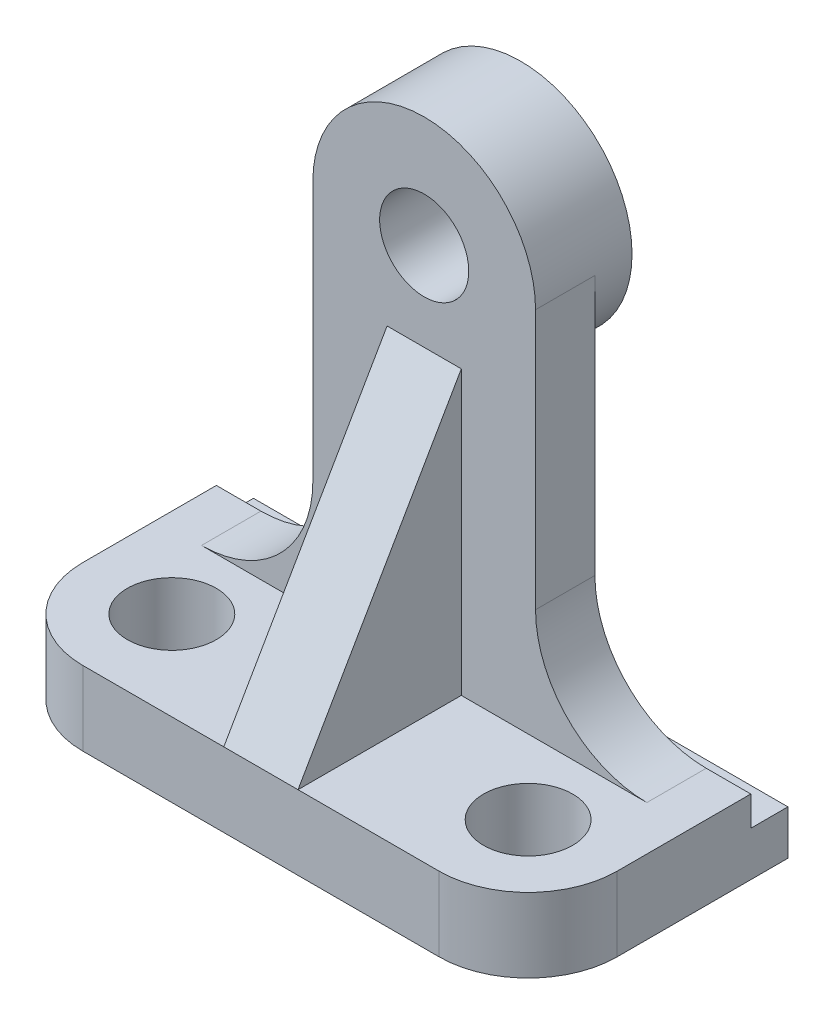
ISO-10303-21;
HEADER;
FILE_DESCRIPTION(('STEP AP214'),'2;1');
FILE_NAME('part.step','',(''),(''),'','','');
FILE_SCHEMA(('AUTOMOTIVE_DESIGN { 1 0 10303 214 1 1 1 1 }'));
ENDSEC;
DATA;
#1=APPLICATION_CONTEXT('core data for automotive mechanical design processes');
#2=APPLICATION_PROTOCOL_DEFINITION('international standard','automotive_design',2000,#1);
#3=PRODUCT_CONTEXT('',#1,'mechanical');
#4=PRODUCT('Part','Part','',(#3));
#5=PRODUCT_RELATED_PRODUCT_CATEGORY('part','',(#4));
#6=PRODUCT_DEFINITION_FORMATION('','',#4);
#7=PRODUCT_DEFINITION_CONTEXT('part definition',#1,'design');
#8=PRODUCT_DEFINITION('design','',#6,#7);
#9=PRODUCT_DEFINITION_SHAPE('','',#8);
#10=(LENGTH_UNIT() NAMED_UNIT(*) SI_UNIT(.MILLI.,.METRE.));
#11=(NAMED_UNIT(*) PLANE_ANGLE_UNIT() SI_UNIT($,.RADIAN.));
#12=(NAMED_UNIT(*) SI_UNIT($,.STERADIAN.) SOLID_ANGLE_UNIT());
#13=UNCERTAINTY_MEASURE_WITH_UNIT(LENGTH_MEASURE(1.E-05),#10,'distance_accuracy_value','');
#14=(GEOMETRIC_REPRESENTATION_CONTEXT(3) GLOBAL_UNCERTAINTY_ASSIGNED_CONTEXT((#13)) GLOBAL_UNIT_ASSIGNED_CONTEXT((#10,
#11,#12)) REPRESENTATION_CONTEXT('',''));
#15=CARTESIAN_POINT('',(0.,0.,0.));
#16=DIRECTION('',(0.,0.,1.));
#17=DIRECTION('',(1.,0.,0.));
#18=AXIS2_PLACEMENT_3D('',#15,#16,#17);
#19=CARTESIAN_POINT('',(23.9999999999999,10.,0.));
#20=DIRECTION('',(0.,-1.,0.));
#21=DIRECTION('',(0.,0.,-1.));
#22=AXIS2_PLACEMENT_3D('',#19,#20,#21);
#23=PLANE('',#22);
#24=CARTESIAN_POINT('',(-24.,10.,0.));
#25=DIRECTION('',(0.,1.,0.));
#26=DIRECTION('',(0.,0.,1.));
#27=AXIS2_PLACEMENT_3D('',#24,#25,#26);
#28=CIRCLE('',#27,6.);
#29=CARTESIAN_POINT('',(-24.,10.,6.));
#30=VERTEX_POINT('',#29);
#31=EDGE_CURVE('E250',#30,#30,#28,.T.);
#32=ORIENTED_EDGE('',*,*,#31,.F.);
#33=EDGE_LOOP('',(#32));
#34=FACE_BOUND('',#33,.T.);
#35=DIRECTION('',(0.,0.,1.));
#36=VECTOR('',#35,1.);
#37=CARTESIAN_POINT('',(-5.,10.,0.));
#38=LINE('',#37,#36);
#39=CARTESIAN_POINT('',(-5.,10.,-10.));
#40=VERTEX_POINT('',#39);
#41=CARTESIAN_POINT('',(-5.,10.,12.));
#42=VERTEX_POINT('',#41);
#43=EDGE_CURVE('E171',#40,#42,#38,.T.);
#44=ORIENTED_EDGE('',*,*,#43,.F.);
#45=DIRECTION('',(1.,0.,0.));
#46=VECTOR('',#45,1.);
#47=CARTESIAN_POINT('',(15.,10.,-10.));
#48=LINE('',#47,#46);
#49=CARTESIAN_POINT('',(-30.,10.,-10.));
#50=VERTEX_POINT('',#49);
#51=EDGE_CURVE('E158',#50,#40,#48,.T.);
#52=ORIENTED_EDGE('',*,*,#51,.F.);
#53=DIRECTION('',(0.,0.,-1.));
#54=VECTOR('',#53,1.);
#55=CARTESIAN_POINT('',(-30.,10.,-18.));
#56=LINE('',#55,#54);
#57=CARTESIAN_POINT('',(-30.,10.,-18.));
#58=VERTEX_POINT('',#57);
#59=EDGE_CURVE('E298',#50,#58,#56,.T.);
#60=ORIENTED_EDGE('',*,*,#59,.T.);
#61=DIRECTION('',(1.,0.,0.));
#62=VECTOR('',#61,1.);
#63=CARTESIAN_POINT('',(-36.,10.,-18.));
#64=LINE('',#63,#62);
#65=CARTESIAN_POINT('',(-36.,10.,-18.));
#66=VERTEX_POINT('',#65);
#67=EDGE_CURVE('E236',#66,#58,#64,.T.);
#68=ORIENTED_EDGE('',*,*,#67,.F.);
#69=DIRECTION('',(0.,0.,1.));
#70=VECTOR('',#69,1.);
#71=CARTESIAN_POINT('',(-36.,10.,-23.));
#72=LINE('',#71,#70);
#73=CARTESIAN_POINT('',(-36.,10.,0.));
#74=VERTEX_POINT('',#73);
#75=EDGE_CURVE('E258',#66,#74,#72,.T.);
#76=ORIENTED_EDGE('',*,*,#75,.T.);
#77=CARTESIAN_POINT('',(-24.,10.,0.));
#78=DIRECTION('',(0.,1.,0.));
#79=DIRECTION('',(0.,0.,-1.));
#80=AXIS2_PLACEMENT_3D('',#77,#78,#79);
#81=CIRCLE('',#80,12.);
#82=CARTESIAN_POINT('',(-24.,10.,12.));
#83=VERTEX_POINT('',#82);
#84=EDGE_CURVE('E259',#74,#83,#81,.T.);
#85=ORIENTED_EDGE('',*,*,#84,.T.);
#86=DIRECTION('',(1.,0.,0.));
#87=VECTOR('',#86,1.);
#88=CARTESIAN_POINT('',(-24.,10.,12.));
#89=LINE('',#88,#87);
#90=EDGE_CURVE('E174',#83,#42,#89,.T.);
#91=ORIENTED_EDGE('',*,*,#90,.T.);
#92=EDGE_LOOP('',(#44,#52,#60,#68,#76,#85,#91));
#93=FACE_BOUND('',#92,.T.);
#94=ADVANCED_FACE('F39',(#34,#93),#23,.F.);
#95=CARTESIAN_POINT('',(24.,10.,0.));
#96=DIRECTION('',(0.,1.,0.));
#97=DIRECTION('',(0.,0.,-1.));
#98=AXIS2_PLACEMENT_3D('',#95,#96,#97);
#99=CIRCLE('',#98,6.);
#100=CARTESIAN_POINT('',(24.,10.,-6.));
#101=VERTEX_POINT('',#100);
#102=EDGE_CURVE('E243',#101,#101,#99,.T.);
#103=ORIENTED_EDGE('',*,*,#102,.F.);
#104=EDGE_LOOP('',(#103));
#105=FACE_BOUND('',#104,.T.);
#106=CARTESIAN_POINT('',(5.,10.,-10.));
#107=VERTEX_POINT('',#106);
#108=CARTESIAN_POINT('',(30.,10.,-10.));
#109=VERTEX_POINT('',#108);
#110=EDGE_CURVE('E168',#107,#109,#48,.T.);
#111=ORIENTED_EDGE('',*,*,#110,.F.);
#112=DIRECTION('',(0.,0.,1.));
#113=VECTOR('',#112,1.);
#114=CARTESIAN_POINT('',(5.,10.,0.));
#115=LINE('',#114,#113);
#116=CARTESIAN_POINT('',(5.,10.,12.));
#117=VERTEX_POINT('',#116);
#118=EDGE_CURVE('E53',#107,#117,#115,.T.);
#119=ORIENTED_EDGE('',*,*,#118,.T.);
#120=CARTESIAN_POINT('',(24.,10.,12.));
#121=VERTEX_POINT('',#120);
#122=EDGE_CURVE('E261',#117,#121,#89,.T.);
#123=ORIENTED_EDGE('',*,*,#122,.T.);
#124=CARTESIAN_POINT('',(23.9999999999999,10.,0.));
#125=DIRECTION('',(0.,1.,0.));
#126=DIRECTION('',(0.,0.,-1.));
#127=AXIS2_PLACEMENT_3D('',#124,#125,#126);
#128=CIRCLE('',#127,12.0000000000001);
#129=CARTESIAN_POINT('',(36.,10.,0.));
#130=VERTEX_POINT('',#129);
#131=EDGE_CURVE('E263',#121,#130,#128,.T.);
#132=ORIENTED_EDGE('',*,*,#131,.T.);
#133=DIRECTION('',(0.,0.,-1.));
#134=VECTOR('',#133,1.);
#135=CARTESIAN_POINT('',(36.,10.,-23.));
#136=LINE('',#135,#134);
#137=CARTESIAN_POINT('',(36.,10.,-18.));
#138=VERTEX_POINT('',#137);
#139=EDGE_CURVE('E251',#130,#138,#136,.T.);
#140=ORIENTED_EDGE('',*,*,#139,.T.);
#141=CARTESIAN_POINT('',(30.,10.,-18.));
#142=VERTEX_POINT('',#141);
#143=EDGE_CURVE('E226',#142,#138,#64,.T.);
#144=ORIENTED_EDGE('',*,*,#143,.F.);
#145=DIRECTION('',(0.,0.,-1.));
#146=VECTOR('',#145,1.);
#147=CARTESIAN_POINT('',(30.,10.,-10.));
#148=LINE('',#147,#146);
#149=EDGE_CURVE('E296',#142,#109,#148,.F.);
#150=ORIENTED_EDGE('',*,*,#149,.T.);
#151=EDGE_LOOP('',(#111,#119,#123,#132,#140,#144,#150));
#152=FACE_BOUND('',#151,.T.);
#153=ADVANCED_FACE('F345',(#105,#152),#23,.F.);
#154=CARTESIAN_POINT('',(23.9999999999999,0.,0.));
#155=DIRECTION('',(0.,-1.,0.));
#156=DIRECTION('',(0.,0.,-1.));
#157=AXIS2_PLACEMENT_3D('',#154,#155,#156);
#158=PLANE('',#157);
#159=CARTESIAN_POINT('',(23.9999999999999,0.,0.));
#160=DIRECTION('',(0.,1.,0.));
#161=DIRECTION('',(0.,0.,-1.));
#162=AXIS2_PLACEMENT_3D('',#159,#160,#161);
#163=CIRCLE('',#162,12.0000000000001);
#164=CARTESIAN_POINT('',(24.,0.,12.));
#165=VERTEX_POINT('',#164);
#166=CARTESIAN_POINT('',(36.,0.,0.));
#167=VERTEX_POINT('',#166);
#168=EDGE_CURVE('E260',#165,#167,#163,.T.);
#169=ORIENTED_EDGE('',*,*,#168,.F.);
#170=DIRECTION('',(1.,0.,0.));
#171=VECTOR('',#170,1.);
#172=CARTESIAN_POINT('',(-24.,0.,12.));
#173=LINE('',#172,#171);
#174=CARTESIAN_POINT('',(-24.,0.,12.));
#175=VERTEX_POINT('',#174);
#176=EDGE_CURVE('E273',#175,#165,#173,.T.);
#177=ORIENTED_EDGE('',*,*,#176,.F.);
#178=CARTESIAN_POINT('',(-24.,0.,0.));
#179=DIRECTION('',(0.,1.,0.));
#180=DIRECTION('',(0.,0.,-1.));
#181=AXIS2_PLACEMENT_3D('',#178,#179,#180);
#182=CIRCLE('',#181,12.);
#183=CARTESIAN_POINT('',(-36.,0.,0.));
#184=VERTEX_POINT('',#183);
#185=EDGE_CURVE('E275',#184,#175,#182,.T.);
#186=ORIENTED_EDGE('',*,*,#185,.F.);
#187=DIRECTION('',(0.,0.,1.));
#188=VECTOR('',#187,1.);
#189=CARTESIAN_POINT('',(-36.,0.,-23.));
#190=LINE('',#189,#188);
#191=CARTESIAN_POINT('',(-36.,0.,-23.));
#192=VERTEX_POINT('',#191);
#193=EDGE_CURVE('E269',#192,#184,#190,.T.);
#194=ORIENTED_EDGE('',*,*,#193,.F.);
#195=DIRECTION('',(-1.,0.,0.));
#196=VECTOR('',#195,1.);
#197=CARTESIAN_POINT('',(-36.,0.,-23.));
#198=LINE('',#197,#196);
#199=CARTESIAN_POINT('',(36.,0.,-23.));
#200=VERTEX_POINT('',#199);
#201=EDGE_CURVE('E268',#200,#192,#198,.T.);
#202=ORIENTED_EDGE('',*,*,#201,.F.);
#203=DIRECTION('',(0.,0.,-1.));
#204=VECTOR('',#203,1.);
#205=CARTESIAN_POINT('',(36.,0.,-23.));
#206=LINE('',#205,#204);
#207=EDGE_CURVE('E249',#167,#200,#206,.T.);
#208=ORIENTED_EDGE('',*,*,#207,.F.);
#209=EDGE_LOOP('',(#169,#177,#186,#194,#202,#208));
#210=FACE_BOUND('',#209,.T.);
#211=CARTESIAN_POINT('',(24.,0.,0.));
#212=DIRECTION('',(0.,1.,0.));
#213=DIRECTION('',(0.,0.,-1.));
#214=AXIS2_PLACEMENT_3D('',#211,#212,#213);
#215=CIRCLE('',#214,6.);
#216=CARTESIAN_POINT('',(24.,0.,-6.));
#217=VERTEX_POINT('',#216);
#218=EDGE_CURVE('E234',#217,#217,#215,.T.);
#219=ORIENTED_EDGE('',*,*,#218,.T.);
#220=EDGE_LOOP('',(#219));
#221=FACE_BOUND('',#220,.T.);
#222=CARTESIAN_POINT('',(-24.,0.,0.));
#223=DIRECTION('',(0.,1.,0.));
#224=DIRECTION('',(0.,0.,1.));
#225=AXIS2_PLACEMENT_3D('',#222,#223,#224);
#226=CIRCLE('',#225,6.);
#227=CARTESIAN_POINT('',(-24.,0.,6.));
#228=VERTEX_POINT('',#227);
#229=EDGE_CURVE('E244',#228,#228,#226,.T.);
#230=ORIENTED_EDGE('',*,*,#229,.T.);
#231=EDGE_LOOP('',(#230));
#232=FACE_BOUND('',#231,.T.);
#233=ADVANCED_FACE('F349',(#210,#221,#232),#158,.T.);
#234=CARTESIAN_POINT('',(36.,10.,-23.));
#235=DIRECTION('',(-1.,0.,0.));
#236=DIRECTION('',(0.,0.,1.));
#237=AXIS2_PLACEMENT_3D('',#234,#235,#236);
#238=PLANE('',#237);
#239=DIRECTION('',(0.,-1.,0.));
#240=VECTOR('',#239,1.);
#241=CARTESIAN_POINT('',(36.,10.,-23.));
#242=LINE('',#241,#240);
#243=CARTESIAN_POINT('',(36.,6.,-23.));
#244=VERTEX_POINT('',#243);
#245=EDGE_CURVE('E292',#244,#200,#242,.T.);
#246=ORIENTED_EDGE('',*,*,#245,.F.);
#247=DIRECTION('',(0.,0.,-1.));
#248=VECTOR('',#247,1.);
#249=CARTESIAN_POINT('',(36.,6.,-18.));
#250=LINE('',#249,#248);
#251=CARTESIAN_POINT('',(36.,6.,-18.));
#252=VERTEX_POINT('',#251);
#253=EDGE_CURVE('E223',#252,#244,#250,.T.);
#254=ORIENTED_EDGE('',*,*,#253,.F.);
#255=DIRECTION('',(0.,-1.,0.));
#256=VECTOR('',#255,1.);
#257=CARTESIAN_POINT('',(36.,10.,-18.));
#258=LINE('',#257,#256);
#259=EDGE_CURVE('E219',#138,#252,#258,.T.);
#260=ORIENTED_EDGE('',*,*,#259,.F.);
#261=ORIENTED_EDGE('',*,*,#139,.F.);
#262=DIRECTION('',(0.,-1.,0.));
#263=VECTOR('',#262,1.);
#264=CARTESIAN_POINT('',(36.,10.,0.));
#265=LINE('',#264,#263);
#266=EDGE_CURVE('E264',#130,#167,#265,.T.);
#267=ORIENTED_EDGE('',*,*,#266,.T.);
#268=ORIENTED_EDGE('',*,*,#207,.T.);
#269=EDGE_LOOP('',(#246,#254,#260,#261,#267,#268));
#270=FACE_BOUND('',#269,.T.);
#271=ADVANCED_FACE('F356',(#270),#238,.F.);
#272=CARTESIAN_POINT('',(-36.,10.,-23.));
#273=DIRECTION('',(0.,0.,1.));
#274=DIRECTION('',(1.,0.,0.));
#275=AXIS2_PLACEMENT_3D('',#272,#273,#274);
#276=PLANE('',#275);
#277=ORIENTED_EDGE('',*,*,#201,.T.);
#278=DIRECTION('',(0.,-1.,0.));
#279=VECTOR('',#278,1.);
#280=CARTESIAN_POINT('',(-36.,10.,-23.));
#281=LINE('',#280,#279);
#282=CARTESIAN_POINT('',(-36.,6.,-23.));
#283=VERTEX_POINT('',#282);
#284=EDGE_CURVE('E287',#283,#192,#281,.T.);
#285=ORIENTED_EDGE('',*,*,#284,.F.);
#286=DIRECTION('',(1.,0.,0.));
#287=VECTOR('',#286,1.);
#288=CARTESIAN_POINT('',(-36.,6.,-23.));
#289=LINE('',#288,#287);
#290=EDGE_CURVE('E232',#283,#244,#289,.T.);
#291=ORIENTED_EDGE('',*,*,#290,.T.);
#292=ORIENTED_EDGE('',*,*,#245,.T.);
#293=EDGE_LOOP('',(#277,#285,#291,#292));
#294=FACE_BOUND('',#293,.T.);
#295=ADVANCED_FACE('F363',(#294),#276,.F.);
#296=CARTESIAN_POINT('',(-36.,10.,-23.));
#297=DIRECTION('',(1.,0.,0.));
#298=DIRECTION('',(0.,0.,-1.));
#299=AXIS2_PLACEMENT_3D('',#296,#297,#298);
#300=PLANE('',#299);
#301=DIRECTION('',(0.,-1.,0.));
#302=VECTOR('',#301,1.);
#303=CARTESIAN_POINT('',(-36.,10.,-18.));
#304=LINE('',#303,#302);
#305=CARTESIAN_POINT('',(-36.,6.,-18.));
#306=VERTEX_POINT('',#305);
#307=EDGE_CURVE('E222',#66,#306,#304,.T.);
#308=ORIENTED_EDGE('',*,*,#307,.T.);
#309=DIRECTION('',(0.,0.,-1.));
#310=VECTOR('',#309,1.);
#311=CARTESIAN_POINT('',(-36.,6.,-18.));
#312=LINE('',#311,#310);
#313=EDGE_CURVE('E221',#306,#283,#312,.T.);
#314=ORIENTED_EDGE('',*,*,#313,.T.);
#315=ORIENTED_EDGE('',*,*,#284,.T.);
#316=ORIENTED_EDGE('',*,*,#193,.T.);
#317=DIRECTION('',(0.,-1.,0.));
#318=VECTOR('',#317,1.);
#319=CARTESIAN_POINT('',(-36.,10.,0.));
#320=LINE('',#319,#318);
#321=EDGE_CURVE('E282',#74,#184,#320,.T.);
#322=ORIENTED_EDGE('',*,*,#321,.F.);
#323=ORIENTED_EDGE('',*,*,#75,.F.);
#324=EDGE_LOOP('',(#308,#314,#315,#316,#322,#323));
#325=FACE_BOUND('',#324,.T.);
#326=ADVANCED_FACE('F318',(#325),#300,.F.);
#327=CARTESIAN_POINT('',(-24.,10.,0.));
#328=DIRECTION('',(0.,-1.,0.));
#329=DIRECTION('',(0.,0.,-1.));
#330=AXIS2_PLACEMENT_3D('',#327,#328,#329);
#331=CYLINDRICAL_SURFACE('',#330,12.);
#332=ORIENTED_EDGE('',*,*,#185,.T.);
#333=DIRECTION('',(0.,-1.,0.));
#334=VECTOR('',#333,1.);
#335=CARTESIAN_POINT('',(-24.,10.,12.));
#336=LINE('',#335,#334);
#337=EDGE_CURVE('E285',#83,#175,#336,.T.);
#338=ORIENTED_EDGE('',*,*,#337,.F.);
#339=ORIENTED_EDGE('',*,*,#84,.F.);
#340=ORIENTED_EDGE('',*,*,#321,.T.);
#341=EDGE_LOOP('',(#332,#338,#339,#340));
#342=FACE_BOUND('',#341,.T.);
#343=ADVANCED_FACE('F322',(#342),#331,.T.);
#344=CARTESIAN_POINT('',(-24.,10.,12.));
#345=DIRECTION('',(0.,0.,-1.));
#346=DIRECTION('',(-1.,0.,0.));
#347=AXIS2_PLACEMENT_3D('',#344,#345,#346);
#348=PLANE('',#347);
#349=ORIENTED_EDGE('',*,*,#122,.F.);
#350=DIRECTION('',(-1.,0.,0.));
#351=VECTOR('',#350,1.);
#352=CARTESIAN_POINT('',(-24.,10.,12.));
#353=LINE('',#352,#351);
#354=EDGE_CURVE('E63',#42,#117,#353,.F.);
#355=ORIENTED_EDGE('',*,*,#354,.F.);
#356=ORIENTED_EDGE('',*,*,#90,.F.);
#357=ORIENTED_EDGE('',*,*,#337,.T.);
#358=ORIENTED_EDGE('',*,*,#176,.T.);
#359=DIRECTION('',(0.,-1.,0.));
#360=VECTOR('',#359,1.);
#361=CARTESIAN_POINT('',(24.,10.,12.));
#362=LINE('',#361,#360);
#363=EDGE_CURVE('E276',#121,#165,#362,.T.);
#364=ORIENTED_EDGE('',*,*,#363,.F.);
#365=EDGE_LOOP('',(#349,#355,#356,#357,#358,#364));
#366=FACE_BOUND('',#365,.T.);
#367=ADVANCED_FACE('F326',(#366),#348,.F.);
#368=CARTESIAN_POINT('',(23.9999999999999,10.,0.));
#369=DIRECTION('',(0.,-1.,0.));
#370=DIRECTION('',(0.,0.,-1.));
#371=AXIS2_PLACEMENT_3D('',#368,#369,#370);
#372=CYLINDRICAL_SURFACE('',#371,12.0000000000001);
#373=ORIENTED_EDGE('',*,*,#168,.T.);
#374=ORIENTED_EDGE('',*,*,#266,.F.);
#375=ORIENTED_EDGE('',*,*,#131,.F.);
#376=ORIENTED_EDGE('',*,*,#363,.T.);
#377=EDGE_LOOP('',(#373,#374,#375,#376));
#378=FACE_BOUND('',#377,.T.);
#379=ADVANCED_FACE('F328',(#378),#372,.T.);
#380=CARTESIAN_POINT('',(-24.,10.,0.));
#381=DIRECTION('',(0.,-1.,0.));
#382=DIRECTION('',(0.,0.,-1.));
#383=AXIS2_PLACEMENT_3D('',#380,#381,#382);
#384=CYLINDRICAL_SURFACE('',#383,6.);
#385=ORIENTED_EDGE('',*,*,#31,.T.);
#386=EDGE_LOOP('',(#385));
#387=FACE_BOUND('',#386,.T.);
#388=ORIENTED_EDGE('',*,*,#229,.F.);
#389=EDGE_LOOP('',(#388));
#390=FACE_BOUND('',#389,.T.);
#391=ADVANCED_FACE('F338',(#387,#390),#384,.F.);
#392=CARTESIAN_POINT('',(24.,10.,0.));
#393=DIRECTION('',(0.,-1.,0.));
#394=DIRECTION('',(0.,0.,-1.));
#395=AXIS2_PLACEMENT_3D('',#392,#393,#394);
#396=CYLINDRICAL_SURFACE('',#395,6.);
#397=ORIENTED_EDGE('',*,*,#102,.T.);
#398=EDGE_LOOP('',(#397));
#399=FACE_BOUND('',#398,.T.);
#400=ORIENTED_EDGE('',*,*,#218,.F.);
#401=EDGE_LOOP('',(#400));
#402=FACE_BOUND('',#401,.T.);
#403=ADVANCED_FACE('F375',(#399,#402),#396,.F.);
#404=CARTESIAN_POINT('',(-36.,6.,-18.));
#405=DIRECTION('',(0.,-1.,0.));
#406=DIRECTION('',(0.,0.,-1.));
#407=AXIS2_PLACEMENT_3D('',#404,#405,#406);
#408=PLANE('',#407);
#409=ORIENTED_EDGE('',*,*,#253,.T.);
#410=ORIENTED_EDGE('',*,*,#290,.F.);
#411=ORIENTED_EDGE('',*,*,#313,.F.);
#412=DIRECTION('',(1.,0.,0.));
#413=VECTOR('',#412,1.);
#414=CARTESIAN_POINT('',(-36.,6.,-18.));
#415=LINE('',#414,#413);
#416=EDGE_CURVE('E237',#306,#252,#415,.T.);
#417=ORIENTED_EDGE('',*,*,#416,.T.);
#418=EDGE_LOOP('',(#409,#410,#411,#417));
#419=FACE_BOUND('',#418,.T.);
#420=ADVANCED_FACE('F380',(#419),#408,.F.);
#421=CARTESIAN_POINT('',(-36.,10.,-18.));
#422=DIRECTION('',(0.,0.,1.));
#423=DIRECTION('',(1.,0.,0.));
#424=AXIS2_PLACEMENT_3D('',#421,#422,#423);
#425=PLANE('',#424);
#426=ORIENTED_EDGE('',*,*,#259,.T.);
#427=ORIENTED_EDGE('',*,*,#416,.F.);
#428=ORIENTED_EDGE('',*,*,#307,.F.);
#429=ORIENTED_EDGE('',*,*,#67,.T.);
#430=CARTESIAN_POINT('',(-30.,25.,-18.));
#431=DIRECTION('',(0.,0.,1.));
#432=DIRECTION('',(1.,0.,0.));
#433=AXIS2_PLACEMENT_3D('',#430,#431,#432);
#434=CIRCLE('',#433,15.);
#435=CARTESIAN_POINT('',(-15.,25.,-18.));
#436=VERTEX_POINT('',#435);
#437=EDGE_CURVE('E50',#58,#436,#434,.T.);
#438=ORIENTED_EDGE('',*,*,#437,.T.);
#439=DIRECTION('',(0.,-1.,0.));
#440=VECTOR('',#439,1.);
#441=CARTESIAN_POINT('',(-15.,10.,-18.));
#442=LINE('',#441,#440);
#443=CARTESIAN_POINT('',(-15.,60.,-18.));
#444=VERTEX_POINT('',#443);
#445=EDGE_CURVE('E215',#444,#436,#442,.T.);
#446=ORIENTED_EDGE('',*,*,#445,.F.);
#447=CARTESIAN_POINT('',(0.,60.,-18.));
#448=DIRECTION('',(0.,0.,1.));
#449=DIRECTION('',(1.,0.,0.));
#450=AXIS2_PLACEMENT_3D('',#447,#448,#449);
#451=CIRCLE('',#450,15.);
#452=CARTESIAN_POINT('',(15.,60.,-18.));
#453=VERTEX_POINT('',#452);
#454=EDGE_CURVE('E203',#444,#453,#451,.T.);
#455=ORIENTED_EDGE('',*,*,#454,.T.);
#456=DIRECTION('',(0.,1.,0.));
#457=VECTOR('',#456,1.);
#458=CARTESIAN_POINT('',(15.,60.,-18.));
#459=LINE('',#458,#457);
#460=CARTESIAN_POINT('',(15.,25.,-18.));
#461=VERTEX_POINT('',#460);
#462=EDGE_CURVE('E204',#461,#453,#459,.T.);
#463=ORIENTED_EDGE('',*,*,#462,.F.);
#464=CARTESIAN_POINT('',(30.,25.,-18.));
#465=DIRECTION('',(0.,0.,1.));
#466=DIRECTION('',(1.,0.,0.));
#467=AXIS2_PLACEMENT_3D('',#464,#465,#466);
#468=CIRCLE('',#467,15.);
#469=EDGE_CURVE('E302',#461,#142,#468,.T.);
#470=ORIENTED_EDGE('',*,*,#469,.T.);
#471=ORIENTED_EDGE('',*,*,#143,.T.);
#472=EDGE_LOOP('',(#426,#427,#428,#429,#438,#446,#455,#463,#470,#471));
#473=FACE_BOUND('',#472,.T.);
#474=ADVANCED_FACE('F306',(#473),#425,.F.);
#475=CARTESIAN_POINT('',(15.,60.,-10.));
#476=DIRECTION('',(-1.,0.,0.));
#477=DIRECTION('',(0.,-1.,0.));
#478=AXIS2_PLACEMENT_3D('',#475,#476,#477);
#479=PLANE('',#478);
#480=DIRECTION('',(0.,1.,0.));
#481=VECTOR('',#480,1.);
#482=CARTESIAN_POINT('',(15.,60.,-10.));
#483=LINE('',#482,#481);
#484=CARTESIAN_POINT('',(15.,25.,-10.));
#485=VERTEX_POINT('',#484);
#486=CARTESIAN_POINT('',(15.,60.,-10.));
#487=VERTEX_POINT('',#486);
#488=EDGE_CURVE('E166',#485,#487,#483,.T.);
#489=ORIENTED_EDGE('',*,*,#488,.F.);
#490=DIRECTION('',(0.,0.,-1.));
#491=VECTOR('',#490,1.);
#492=CARTESIAN_POINT('',(15.,25.,-18.));
#493=LINE('',#492,#491);
#494=EDGE_CURVE('E291',#485,#461,#493,.T.);
#495=ORIENTED_EDGE('',*,*,#494,.T.);
#496=ORIENTED_EDGE('',*,*,#462,.T.);
#497=DIRECTION('',(0.,0.,-1.));
#498=VECTOR('',#497,1.);
#499=CARTESIAN_POINT('',(15.,60.,-10.));
#500=LINE('',#499,#498);
#501=EDGE_CURVE('E220',#487,#453,#500,.T.);
#502=ORIENTED_EDGE('',*,*,#501,.F.);
#503=EDGE_LOOP('',(#489,#495,#496,#502));
#504=FACE_BOUND('',#503,.T.);
#505=ADVANCED_FACE('F387',(#504),#479,.F.);
#506=CARTESIAN_POINT('',(-15.,10.,-10.));
#507=DIRECTION('',(1.,0.,0.));
#508=DIRECTION('',(0.,0.,-1.));
#509=AXIS2_PLACEMENT_3D('',#506,#507,#508);
#510=PLANE('',#509);
#511=ORIENTED_EDGE('',*,*,#445,.T.);
#512=DIRECTION('',(0.,0.,-1.));
#513=VECTOR('',#512,1.);
#514=CARTESIAN_POINT('',(-15.,25.,-10.));
#515=LINE('',#514,#513);
#516=CARTESIAN_POINT('',(-15.,25.,-10.));
#517=VERTEX_POINT('',#516);
#518=EDGE_CURVE('E301',#436,#517,#515,.F.);
#519=ORIENTED_EDGE('',*,*,#518,.T.);
#520=DIRECTION('',(0.,-1.,0.));
#521=VECTOR('',#520,1.);
#522=CARTESIAN_POINT('',(-15.,10.,-10.));
#523=LINE('',#522,#521);
#524=CARTESIAN_POINT('',(-15.,60.,-10.));
#525=VERTEX_POINT('',#524);
#526=EDGE_CURVE('E210',#525,#517,#523,.T.);
#527=ORIENTED_EDGE('',*,*,#526,.F.);
#528=DIRECTION('',(0.,0.,-1.));
#529=VECTOR('',#528,1.);
#530=CARTESIAN_POINT('',(-15.,60.,-10.));
#531=LINE('',#530,#529);
#532=EDGE_CURVE('E207',#525,#444,#531,.T.);
#533=ORIENTED_EDGE('',*,*,#532,.T.);
#534=EDGE_LOOP('',(#511,#519,#527,#533));
#535=FACE_BOUND('',#534,.T.);
#536=ADVANCED_FACE('F311',(#535),#510,.F.);
#537=CARTESIAN_POINT('',(0.,0.,-10.));
#538=DIRECTION('',(0.,0.,-1.));
#539=DIRECTION('',(-1.,0.,0.));
#540=AXIS2_PLACEMENT_3D('',#537,#538,#539);
#541=PLANE('',#540);
#542=CARTESIAN_POINT('',(0.,60.,-10.));
#543=DIRECTION('',(0.,0.,1.));
#544=DIRECTION('',(1.,0.,0.));
#545=AXIS2_PLACEMENT_3D('',#542,#543,#544);
#546=CIRCLE('',#545,6.);
#547=CARTESIAN_POINT('',(6.,60.,-10.));
#548=VERTEX_POINT('',#547);
#549=EDGE_CURVE('E191',#548,#548,#546,.T.);
#550=ORIENTED_EDGE('',*,*,#549,.F.);
#551=EDGE_LOOP('',(#550));
#552=FACE_BOUND('',#551,.T.);
#553=DIRECTION('',(-1.,0.,0.));
#554=VECTOR('',#553,1.);
#555=CARTESIAN_POINT('',(0.,48.1051177665149,-10.));
#556=LINE('',#555,#554);
#557=CARTESIAN_POINT('',(-5.,48.1051177665149,-10.));
#558=VERTEX_POINT('',#557);
#559=CARTESIAN_POINT('',(5.,48.1051177665149,-10.));
#560=VERTEX_POINT('',#559);
#561=EDGE_CURVE('E186',#558,#560,#556,.F.);
#562=ORIENTED_EDGE('',*,*,#561,.T.);
#563=DIRECTION('',(0.,-1.,0.));
#564=VECTOR('',#563,1.);
#565=CARTESIAN_POINT('',(5.,0.,-10.));
#566=LINE('',#565,#564);
#567=EDGE_CURVE('E181',#560,#107,#566,.T.);
#568=ORIENTED_EDGE('',*,*,#567,.T.);
#569=ORIENTED_EDGE('',*,*,#110,.T.);
#570=CARTESIAN_POINT('',(30.,25.,-10.));
#571=DIRECTION('',(0.,0.,-1.));
#572=DIRECTION('',(-1.,0.,0.));
#573=AXIS2_PLACEMENT_3D('',#570,#571,#572);
#574=CIRCLE('',#573,15.);
#575=EDGE_CURVE('E304',#109,#485,#574,.T.);
#576=ORIENTED_EDGE('',*,*,#575,.T.);
#577=ORIENTED_EDGE('',*,*,#488,.T.);
#578=CARTESIAN_POINT('',(0.,60.,-10.));
#579=DIRECTION('',(0.,0.,1.));
#580=DIRECTION('',(1.,0.,0.));
#581=AXIS2_PLACEMENT_3D('',#578,#579,#580);
#582=CIRCLE('',#581,15.);
#583=EDGE_CURVE('E194',#487,#525,#582,.T.);
#584=ORIENTED_EDGE('',*,*,#583,.T.);
#585=ORIENTED_EDGE('',*,*,#526,.T.);
#586=CARTESIAN_POINT('',(-30.,25.,-10.));
#587=DIRECTION('',(0.,0.,-1.));
#588=DIRECTION('',(-1.,0.,0.));
#589=AXIS2_PLACEMENT_3D('',#586,#587,#588);
#590=CIRCLE('',#589,15.);
#591=EDGE_CURVE('E11',#517,#50,#590,.T.);
#592=ORIENTED_EDGE('',*,*,#591,.T.);
#593=ORIENTED_EDGE('',*,*,#51,.T.);
#594=DIRECTION('',(0.,-1.,0.));
#595=VECTOR('',#594,1.);
#596=CARTESIAN_POINT('',(-5.,0.,-10.));
#597=LINE('',#596,#595);
#598=EDGE_CURVE('E165',#558,#40,#597,.T.);
#599=ORIENTED_EDGE('',*,*,#598,.F.);
#600=EDGE_LOOP('',(#562,#568,#569,#576,#577,#584,#585,#592,#593,#599));
#601=FACE_BOUND('',#600,.T.);
#602=ADVANCED_FACE('F159',(#552,#601),#541,.F.);
#603=CARTESIAN_POINT('',(0.,60.,-23.));
#604=DIRECTION('',(0.,0.,1.));
#605=DIRECTION('',(1.,0.,0.));
#606=AXIS2_PLACEMENT_3D('',#603,#604,#605);
#607=CYLINDRICAL_SURFACE('',#606,15.);
#608=ORIENTED_EDGE('',*,*,#501,.T.);
#609=ORIENTED_EDGE('',*,*,#454,.F.);
#610=ORIENTED_EDGE('',*,*,#532,.F.);
#611=ORIENTED_EDGE('',*,*,#583,.F.);
#612=EDGE_LOOP('',(#608,#609,#610,#611));
#613=FACE_BOUND('',#612,.T.);
#614=CARTESIAN_POINT('',(0.,60.,-23.));
#615=DIRECTION('',(0.,0.,1.));
#616=DIRECTION('',(1.,0.,0.));
#617=AXIS2_PLACEMENT_3D('',#614,#615,#616);
#618=CIRCLE('',#617,15.);
#619=CARTESIAN_POINT('',(15.,60.,-23.));
#620=VERTEX_POINT('',#619);
#621=EDGE_CURVE('E196',#620,#620,#618,.T.);
#622=ORIENTED_EDGE('',*,*,#621,.T.);
#623=EDGE_LOOP('',(#622));
#624=FACE_BOUND('',#623,.T.);
#625=ADVANCED_FACE('F392',(#613,#624),#607,.T.);
#626=CARTESIAN_POINT('',(0.,60.,-23.));
#627=DIRECTION('',(0.,0.,1.));
#628=DIRECTION('',(1.,0.,0.));
#629=AXIS2_PLACEMENT_3D('',#626,#627,#628);
#630=CYLINDRICAL_SURFACE('',#629,6.);
#631=CARTESIAN_POINT('',(0.,60.,-23.));
#632=DIRECTION('',(0.,0.,1.));
#633=DIRECTION('',(1.,0.,0.));
#634=AXIS2_PLACEMENT_3D('',#631,#632,#633);
#635=CIRCLE('',#634,6.);
#636=CARTESIAN_POINT('',(6.,60.,-23.));
#637=VERTEX_POINT('',#636);
#638=EDGE_CURVE('E195',#637,#637,#635,.T.);
#639=CARTESIAN_POINT('',(6.,60.,-23.));
#640=CARTESIAN_POINT('',(6.,60.,-22.8645833333333));
#641=CARTESIAN_POINT('',(6.,60.,-22.7291666666667));
#642=CARTESIAN_POINT('',(6.,60.,-22.4583333333333));
#643=CARTESIAN_POINT('',(6.,60.,-22.3229166666667));
#644=CARTESIAN_POINT('',(6.,60.,-22.0520833333333));
#645=CARTESIAN_POINT('',(6.,60.,-21.9166666666667));
#646=CARTESIAN_POINT('',(6.,60.,-21.6458333333333));
#647=CARTESIAN_POINT('',(6.,60.,-21.5104166666667));
#648=CARTESIAN_POINT('',(6.,60.,-21.2395833333333));
#649=CARTESIAN_POINT('',(6.,60.,-21.1041666666667));
#650=CARTESIAN_POINT('',(6.,60.,-20.8333333333333));
#651=CARTESIAN_POINT('',(6.,60.,-20.6979166666667));
#652=CARTESIAN_POINT('',(6.,60.,-20.4270833333333));
#653=CARTESIAN_POINT('',(6.,60.,-20.2916666666667));
#654=CARTESIAN_POINT('',(6.,60.,-20.0208333333333));
#655=CARTESIAN_POINT('',(6.,60.,-19.8854166666667));
#656=CARTESIAN_POINT('',(6.,60.,-19.6145833333333));
#657=CARTESIAN_POINT('',(6.,60.,-19.4791666666667));
#658=CARTESIAN_POINT('',(6.,60.,-19.2083333333333));
#659=CARTESIAN_POINT('',(6.,60.,-19.0729166666667));
#660=CARTESIAN_POINT('',(6.,60.,-18.8020833333333));
#661=CARTESIAN_POINT('',(6.,60.,-18.6666666666667));
#662=CARTESIAN_POINT('',(6.,60.,-18.3958333333333));
#663=CARTESIAN_POINT('',(6.,60.,-18.2604166666667));
#664=CARTESIAN_POINT('',(6.,60.,-17.9895833333333));
#665=CARTESIAN_POINT('',(6.,60.,-17.8541666666667));
#666=CARTESIAN_POINT('',(6.,60.,-17.5833333333333));
#667=CARTESIAN_POINT('',(6.,60.,-17.4479166666667));
#668=CARTESIAN_POINT('',(6.,60.,-17.1770833333333));
#669=CARTESIAN_POINT('',(6.,60.,-17.0416666666667));
#670=CARTESIAN_POINT('',(6.,60.,-16.7708333333333));
#671=CARTESIAN_POINT('',(6.,60.,-16.6354166666667));
#672=CARTESIAN_POINT('',(6.,60.,-16.3645833333333));
#673=CARTESIAN_POINT('',(6.,60.,-16.2291666666667));
#674=CARTESIAN_POINT('',(6.,60.,-15.9583333333333));
#675=CARTESIAN_POINT('',(6.,60.,-15.8229166666667));
#676=CARTESIAN_POINT('',(6.,60.,-15.5520833333333));
#677=CARTESIAN_POINT('',(6.,60.,-15.4166666666667));
#678=CARTESIAN_POINT('',(6.,60.,-15.1458333333333));
#679=CARTESIAN_POINT('',(6.,60.,-15.0104166666667));
#680=CARTESIAN_POINT('',(6.,60.,-14.7395833333333));
#681=CARTESIAN_POINT('',(6.,60.,-14.6041666666667));
#682=CARTESIAN_POINT('',(6.,60.,-14.3333333333333));
#683=CARTESIAN_POINT('',(6.,60.,-14.1979166666667));
#684=CARTESIAN_POINT('',(6.,60.,-13.9270833333333));
#685=CARTESIAN_POINT('',(6.,60.,-13.7916666666667));
#686=CARTESIAN_POINT('',(6.,60.,-13.5208333333333));
#687=CARTESIAN_POINT('',(6.,60.,-13.3854166666667));
#688=CARTESIAN_POINT('',(6.,60.,-13.1145833333333));
#689=CARTESIAN_POINT('',(6.,60.,-12.9791666666667));
#690=CARTESIAN_POINT('',(6.,60.,-12.7083333333333));
#691=CARTESIAN_POINT('',(6.,60.,-12.5729166666667));
#692=CARTESIAN_POINT('',(6.,60.,-12.3020833333333));
#693=CARTESIAN_POINT('',(6.,60.,-12.1666666666667));
#694=CARTESIAN_POINT('',(6.,60.,-11.8958333333333));
#695=CARTESIAN_POINT('',(6.,60.,-11.7604166666667));
#696=CARTESIAN_POINT('',(6.,60.,-11.4895833333333));
#697=CARTESIAN_POINT('',(6.,60.,-11.3541666666667));
#698=CARTESIAN_POINT('',(6.,60.,-11.0833333333333));
#699=CARTESIAN_POINT('',(6.,60.,-10.9479166666667));
#700=CARTESIAN_POINT('',(6.,60.,-10.6770833333333));
#701=CARTESIAN_POINT('',(6.,60.,-10.5416666666667));
#702=CARTESIAN_POINT('',(6.,60.,-10.2708333333333));
#703=CARTESIAN_POINT('',(6.,60.,-10.1354166666667));
#704=CARTESIAN_POINT('',(6.,60.,-10.));
#705=B_SPLINE_CURVE_WITH_KNOTS('',3,(#639,#640,#641,#642,#643,#644,#645,#646,#647,#648,#649,
#650,#651,#652,#653,#654,#655,#656,#657,#658,#659,#660,#661,#662,#663,#664,#665,#666,#667,#668,
#669,#670,#671,#672,#673,#674,#675,#676,#677,#678,#679,#680,#681,#682,#683,#684,#685,#686,#687,
#688,#689,#690,#691,#692,#693,#694,#695,#696,#697,#698,#699,#700,#701,#702,#703,#704),
.UNSPECIFIED.,.F.,.F.,(4,2,2,2,2,2,2,2,2,2,2,2,2,2,2,2,2,2,2,2,2,2,2,2,2,2,2,2,2,2,2,2,4),(0.,
0.40625,0.812500000000001,1.21875,1.625,2.03125,2.4375,2.84375,3.25,3.65625,4.0625,4.46875,
4.875,5.28125,5.6875,6.09375,6.5,6.90625,7.3125,7.71875,8.125,8.53125,8.9375,9.34375,9.75,
10.15625,10.5625,10.96875,11.375,11.78125,12.1875,12.59375,13.),.UNSPECIFIED.);
#706=EDGE_CURVE('BSEAM398',#637,#548,#705,.T.);
#707=ORIENTED_EDGE('',*,*,#638,.F.);
#708=ORIENTED_EDGE('',*,*,#549,.T.);
#709=ORIENTED_EDGE('',*,*,#706,.T.);
#710=ORIENTED_EDGE('',*,*,#706,.F.);
#711=EDGE_LOOP('',(#707,#709,#708,#710));
#712=FACE_BOUND('',#711,.T.);
#713=ADVANCED_FACE('F398',(#712),#630,.F.);
#714=CARTESIAN_POINT('',(0.,60.,-23.));
#715=DIRECTION('',(0.,0.,1.));
#716=DIRECTION('',(1.,0.,0.));
#717=AXIS2_PLACEMENT_3D('',#714,#715,#716);
#718=PLANE('',#717);
#719=ORIENTED_EDGE('',*,*,#638,.T.);
#720=EDGE_LOOP('',(#719));
#721=FACE_BOUND('',#720,.T.);
#722=ORIENTED_EDGE('',*,*,#621,.F.);
#723=EDGE_LOOP('',(#722));
#724=FACE_BOUND('',#723,.T.);
#725=ADVANCED_FACE('F402',(#721,#724),#718,.F.);
#726=CARTESIAN_POINT('',(30.,25.,-10.));
#727=DIRECTION('',(0.,0.,1.));
#728=DIRECTION('',(1.,0.,0.));
#729=AXIS2_PLACEMENT_3D('',#726,#727,#728);
#730=CYLINDRICAL_SURFACE('',#729,15.);
#731=ORIENTED_EDGE('',*,*,#575,.F.);
#732=ORIENTED_EDGE('',*,*,#149,.F.);
#733=ORIENTED_EDGE('',*,*,#469,.F.);
#734=ORIENTED_EDGE('',*,*,#494,.F.);
#735=EDGE_LOOP('',(#731,#732,#733,#734));
#736=FACE_BOUND('',#735,.T.);
#737=ADVANCED_FACE('F404',(#736),#730,.F.);
#738=CARTESIAN_POINT('',(-30.,25.,0.));
#739=DIRECTION('',(0.,0.,1.));
#740=DIRECTION('',(1.,0.,0.));
#741=AXIS2_PLACEMENT_3D('',#738,#739,#740);
#742=CYLINDRICAL_SURFACE('',#741,15.);
#743=ORIENTED_EDGE('',*,*,#591,.F.);
#744=ORIENTED_EDGE('',*,*,#518,.F.);
#745=ORIENTED_EDGE('',*,*,#437,.F.);
#746=ORIENTED_EDGE('',*,*,#59,.F.);
#747=EDGE_LOOP('',(#743,#744,#745,#746));
#748=FACE_BOUND('',#747,.T.);
#749=ADVANCED_FACE('F41',(#748),#742,.F.);
#750=CARTESIAN_POINT('',(0.,10.,12.));
#751=DIRECTION('',(0.,-0.500000000000004,-0.866025403784436));
#752=DIRECTION('',(0.,0.866025403784436,-0.500000000000004));
#753=AXIS2_PLACEMENT_3D('',#750,#751,#752);
#754=PLANE('',#753);
#755=DIRECTION('',(0.,0.866025403784436,-0.500000000000004));
#756=VECTOR('',#755,1.);
#757=CARTESIAN_POINT('',(-5.,10.,12.));
#758=LINE('',#757,#756);
#759=EDGE_CURVE('E182',#42,#558,#758,.T.);
#760=ORIENTED_EDGE('',*,*,#759,.F.);
#761=ORIENTED_EDGE('',*,*,#354,.T.);
#762=DIRECTION('',(0.,0.866025403784436,-0.500000000000004));
#763=VECTOR('',#762,1.);
#764=CARTESIAN_POINT('',(5.,10.,12.));
#765=LINE('',#764,#763);
#766=EDGE_CURVE('E177',#117,#560,#765,.T.);
#767=ORIENTED_EDGE('',*,*,#766,.T.);
#768=ORIENTED_EDGE('',*,*,#561,.F.);
#769=EDGE_LOOP('',(#760,#761,#767,#768));
#770=FACE_BOUND('',#769,.T.);
#771=ADVANCED_FACE('F409',(#770),#754,.F.);
#772=CARTESIAN_POINT('',(5.,37.5,-5.5));
#773=DIRECTION('',(1.,0.,0.));
#774=DIRECTION('',(0.,0.,-1.));
#775=AXIS2_PLACEMENT_3D('',#772,#773,#774);
#776=PLANE('',#775);
#777=ORIENTED_EDGE('',*,*,#567,.F.);
#778=ORIENTED_EDGE('',*,*,#766,.F.);
#779=ORIENTED_EDGE('',*,*,#118,.F.);
#780=EDGE_LOOP('',(#777,#778,#779));
#781=FACE_BOUND('',#780,.T.);
#782=ADVANCED_FACE('F415',(#781),#776,.T.);
#783=CARTESIAN_POINT('',(-5.,37.5,-5.5));
#784=DIRECTION('',(1.,0.,0.));
#785=DIRECTION('',(0.,0.,-1.));
#786=AXIS2_PLACEMENT_3D('',#783,#784,#785);
#787=PLANE('',#786);
#788=ORIENTED_EDGE('',*,*,#759,.T.);
#789=ORIENTED_EDGE('',*,*,#598,.T.);
#790=ORIENTED_EDGE('',*,*,#43,.T.);
#791=EDGE_LOOP('',(#788,#789,#790));
#792=FACE_BOUND('',#791,.T.);
#793=ADVANCED_FACE('F179',(#792),#787,.F.);
#794=CLOSED_SHELL('',(#94,#153,#233,#271,#295,#326,#343,#367,#379,#391,#403,#420,#474,#505,#536,
#602,#625,#713,#725,#737,#749,#771,#782,#793));
#795=MANIFOLD_SOLID_BREP('B2',#794);
#796=ADVANCED_BREP_SHAPE_REPRESENTATION('',(#18,#795),#14);
#797=SHAPE_DEFINITION_REPRESENTATION(#9,#796);
ENDSEC;
END-ISO-10303-21;
